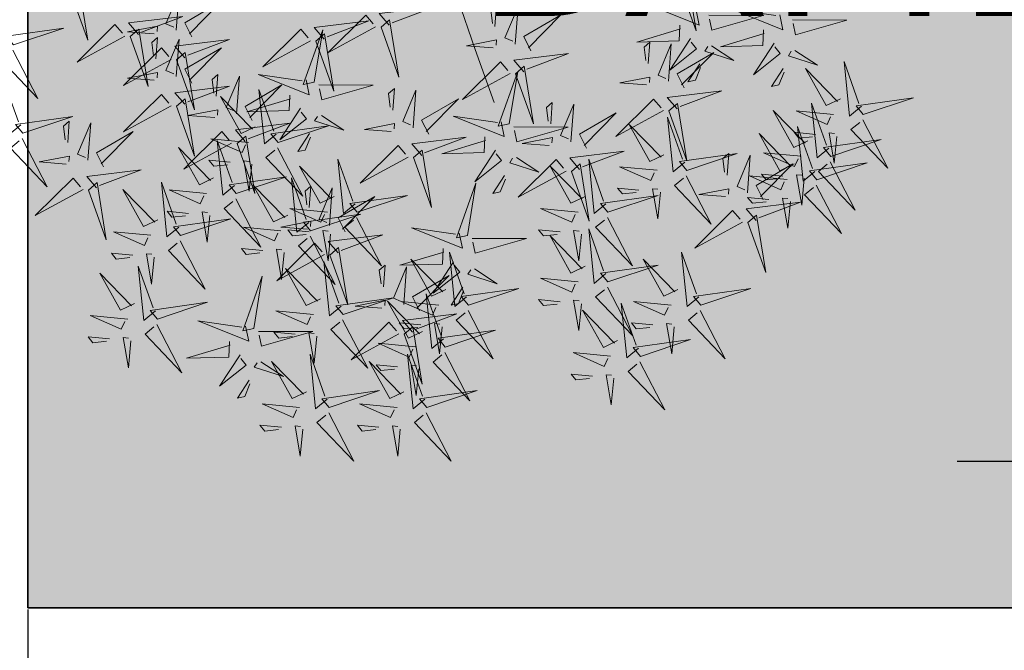
# Model space of a CAD drawing. Units: inches. Extents: x 1704 to 6393, y -157 to 1172.
# Tile 3 of 122: x 1898 to 1933, y -5 to 17. Entities that reach past the tile are written whole.
import ezdxf

# ---------------------------------------------------------------- set-up
doc = ezdxf.new("R2010")
doc.units = ezdxf.units.IN
doc.header["$MEASUREMENT"] = 0
for name, color, linetype, lineweight in [('A-ANNO-DIMS', 7, 'Continuous', 13), ('C-PROP', 7, 'Continuous', 35), ('L-shrub', 74, 'Continuous', 18), ('L-tree', 102, 'Continuous', 18)]:
    doc.layers.add(name, color=color, linetype=linetype, lineweight=lineweight)
doc.layers.add('L-PLNT-PATT', color=253, linetype='Continuous', lineweight=13, true_color=0x9abc8f)
doc.styles.get("Standard").update_dxf_attribs({"font": 'arial.ttf'})
doc.dimstyles.get("Standard").update_dxf_attribs({"dimtxt": 6, "dimasz": 2, "dimexe": 0.18, "dimexo": 0.0625, "dimgap": 0.09, "dimtad": 0, "dimtih": 1, "dimtoh": 1, "dimdec": 1, "dimzin": 0, "dimdsep": 46, "dimlunit": 3, "dimtxsty": 'Standard', "dimblk": 'ARCHTICK', "dimcen": 0.09, "dimadec": 0, "dimazin": 0, "dimtfac": 1, "dimtdec": 1, "dimtofl": 0, "dimtmove": 0, "dimatfit": 3, "dimfxl": 1, "dimtolj": 1, "dimtzin": 0, "dimarcsym": 0})

# ---------------------------------------------------------------- blocks, each defined once
blk = doc.blocks.new('bamboo')
blk.add_line((390, 162.3), (546.4, 218.1))
at = {"layer": 'L-shrub'}
blk.add_line((32.3, 39.5), (390, 162.3), dxfattribs=at)
for points in [[(581.6, 1302), (532.2, 1449.6), (555.7, 1280.7), (581.6, 1302)], [(597.3, 1300.4), (739.2, 1374), (625.7, 1265.9), (604.4, 1291.8)], [(704.4, 1206.5), (655.1, 1354.1), (678.6, 1185.2), (704.4, 1206.5)], [(772.7, 1165.6), (723.3, 1313.2), (746.9, 1144.3), (772.7, 1165.6)], [(557.2, 1296.4), (585.7, 1261.9), (425.4, 1245.7), (548.6, 1289.3)], [(720.2, 1205), (862.1, 1278.5), (748.6, 1170.5), (727.3, 1196.4)], [(303.5, 1094), (304.2, 1253.9), (347.3, 1103.2), (314.4, 1096.3)], [(535.5, 1235), (555.3, 1193.4), (446.4, 1132.5), (542.6, 1226.4)], [(581.2, 1214.7), (570.7, 1104.6), (611.1, 1195.9), (588.3, 1206.1)], [(645.6, 1224.3), (724.2, 1216.7), (635.4, 1201.5), (637, 1217.2)], [(788.4, 1164.1), (930.3, 1237.6), (816.9, 1129.6), (795.5, 1155.5)], [(680.1, 1200.9), (708.6, 1166.4), (548.3, 1150.2), (671.5, 1193.8)], [(393.3, 1101.5), (436.5, 1167.6), (408.8, 1082), (395.6, 1090.6)], [(748.4, 1160), (776.8, 1125.5), (616.6, 1109.3), (739.8, 1152.9)], [(639.6, 1161.5), (633.5, 1098.6), (650.8, 1112.8), (646.7, 1152.8)], [(658.4, 1139.6), (678.2, 1098), (569.2, 1037.1), (665.5, 1130.9)], [(768.4, 1128.9), (847.1, 1121.3), (758.3, 1106.1), (759.8, 1121.8)], [(726.6, 1098.6), (746.5, 1057), (637.5, 996.2), (733.8, 1090)], [(704, 1119.3), (693.5, 1009.2), (734, 1100.5), (711.2, 1110.6)], [(892.5, 987.3), (858.6, 958.2), (839.1, 1118), (885.2, 995.8)], [(830.7, 1007.8), (789.5, 987.1), (726.4, 1094.8), (822.2, 1000.5)], [(772.3, 1078.4), (761.8, 968.3), (802.3, 1059.6), (779.4, 1069.7)], [(836.7, 1088), (915.3, 1080.4), (826.6, 1065.2), (828.1, 1080.9)], [(288.5, 1056.7), (332.3, 1065.9), (272.3, 916.4), (290.8, 1045.7)], [(372, 1040), (464.6, 979.6), (402.5, 1057.8), (382.9, 1042.3)], [(446.2, 1067), (499.2, 1032.5), (494.6, 1054.4), (457.2, 1069.3)], [(762.4, 1066), (756.4, 1003.1), (773.6, 1017.3), (769.5, 1057.4)], [(830.7, 1025.1), (824.7, 962.2), (841.9, 976.4), (837.8, 1016.5)], [(898.5, 963.1), (1045.1, 1015.5), (876.7, 988.5), (898.5, 963.1)], [(289.9, 848.6), (290.5, 1008.4), (333.6, 857.8), (300.8, 850.9)], [(332.8, 1008.9), (378.9, 1007.2), (382.3, 882.5), (343.8, 1011.2)], [(811.3, 961.7), (701, 970), (793.1, 931.4), (802.8, 954.4)], [(1141.3, 824.7), (1092, 972.3), (1115.5, 803.4), (1141.3, 824.7)], [(745.4, 783.8), (696, 931.4), (719.6, 762.5), (745.4, 783.8)], [(897.3, 947.3), (973.8, 807), (863.4, 918.2), (888.9, 940.1)], [(379.6, 856.1), (422.9, 922.2), (395.2, 836.5), (381.9, 845.1)], [(759.2, 902.3), (696.2, 907), (710.8, 890.1), (750.8, 895)], [(822.2, 897.5), (816.2, 818.8), (799.2, 907.2), (815, 906)], [(1157.1, 823.2), (1299, 896.7), (1185.5, 788.7), (1164.2, 814.6)], [(564.8, 755.5), (530.9, 726.4), (511.4, 886.2), (557.5, 764)], [(503, 776), (461.8, 755.3), (398.7, 863), (494.5, 768.7)], [(761.1, 782.3), (903, 855.8), (789.6, 747.8), (768.2, 773.7)], [(188.6, 758.6), (335.2, 810.9), (166.8, 784), (188.6, 758.6)], [(274.9, 811.2), (318.6, 820.4), (258.7, 670.9), (277.2, 800.3)], [(358.3, 794.5), (451, 734.2), (388.8, 812.4), (369.3, 796.8)], [(432.6, 821.6), (485.5, 787.1), (480.9, 808.9), (443.5, 823.9)], [(1117, 819.1), (1145.4, 784.6), (985.2, 768.4), (1108.4, 812)], [(570.9, 731.3), (717.4, 783.7), (549, 756.7), (570.9, 731.3)], [(1291.5, 647.4), (1242.1, 795), (1265.7, 626.1), (1291.5, 647.4)], [(319.2, 763.5), (365.2, 761.8), (368.6, 637), (330.1, 765.8)], [(721.1, 778.2), (749.5, 743.7), (589.3, 727.5), (712.5, 771.1)], [(1095.3, 757.7), (1115.1, 716.2), (1006.1, 655.3), (1102.4, 749.1)], [(483.6, 729.9), (373.4, 738.2), (465.5, 699.6), (475.2, 722.6)], [(1140.9, 737.5), (1130.4, 627.4), (1170.9, 718.7), (1148, 728.8)], [(1205.3, 747.1), (1283.9, 739.5), (1195.2, 724.3), (1196.7, 740)], [(569.7, 715.5), (646.1, 575.2), (535.8, 686.4), (561.2, 708.3)], [(699.3, 716.8), (719.2, 675.2), (610.2, 614.4), (706.4, 708.2)], [(745, 696.6), (734.5, 586.5), (774.9, 677.8), (752.1, 687.9)], [(809.4, 706.2), (888, 698.6), (799.3, 683.4), (800.8, 699.1)], [(868.3, 552), (818.9, 699.6), (842.4, 530.7), (868.3, 552)], [(1073.1, 552), (1023.7, 699.6), (1047.2, 530.7), (1073.1, 552)], [(1307.2, 645.9), (1449.1, 719.5), (1335.7, 611.4), (1314.3, 637.3)], [(431.6, 670.5), (368.6, 675.2), (383.1, 658.2), (423.1, 663.2)], [(494.6, 665.7), (488.6, 587), (471.6, 675.4), (487.3, 674.2)], [(1199.3, 684.2), (1193.3, 621.3), (1210.5, 635.5), (1206.4, 675.6)], [(803.4, 643.3), (797.4, 580.4), (814.6, 594.6), (810.5, 634.7)], [(1267.2, 641.9), (1295.6, 607.4), (1135.4, 591.1), (1258.6, 634.8)], [(884, 550.5), (1025.9, 624), (912.4, 516), (891.1, 541.8)], [(1088.8, 550.5), (1230.7, 624), (1117.2, 516), (1095.9, 541.8)], [(742.3, 469.2), (708.4, 440), (688.9, 599.9), (735, 477.6)], [(1245.4, 580.5), (1265.3, 538.9), (1156.3, 478), (1252.6, 571.9)], [(680.5, 489.6), (639.3, 469), (576.2, 576.7), (672, 482.3)], [(1291.1, 560.2), (1280.6, 450.1), (1321.1, 541.4), (1298.2, 551.6)], [(1355.5, 569.8), (1434.1, 562.2), (1345.4, 547), (1346.9, 562.7)], [(843.9, 546.4), (872.4, 511.9), (712.1, 495.7), (835.3, 539.3)], [(1048.7, 546.4), (1077.2, 511.9), (916.9, 495.7), (1040.1, 539.3)], [(748.4, 444.9), (894.9, 497.3), (726.5, 470.3), (748.4, 444.9)], [(1349.5, 506.9), (1343.5, 444), (1360.7, 458.2), (1356.6, 498.3)], [(822.2, 485), (842, 443.4), (733.1, 382.6), (829.3, 476.4)], [(867.9, 464.7), (857.4, 354.7), (897.8, 446), (875, 456.1)], [(932.3, 474.4), (1010.9, 466.8), (922.2, 451.6), (923.7, 467.3)], [(1027, 485), (1046.8, 443.4), (937.9, 382.6), (1034.1, 476.4)], [(1072.7, 464.7), (1062.1, 354.7), (1102.6, 446), (1079.8, 456.1)], [(1137.1, 474.4), (1215.7, 466.8), (1126.9, 451.6), (1128.4, 467.3)], [(455.6, 305.5), (421.7, 276.4), (402.2, 436.3), (448.3, 314)], [(661.1, 443.6), (550.9, 451.8), (643, 413.2), (652.6, 436.3)], [(617.5, 275.9), (618.2, 435.7), (661.3, 285.1), (628.5, 278.2)], [(393.8, 326), (352.6, 305.3), (289.5, 413), (385.3, 318.7)], [(747.2, 429.2), (823.6, 288.8), (713.3, 400), (738.7, 421.9)], [(926.3, 411.5), (920.3, 348.6), (937.5, 362.8), (933.4, 402.9)], [(1131.1, 411.5), (1125, 348.6), (1142.3, 362.8), (1138.2, 402.9)], [(609.1, 384.1), (546.1, 388.8), (560.6, 371.9), (600.6, 376.8)], [(672.1, 379.4), (666.1, 300.6), (649, 389), (664.8, 387.8)], [(707.3, 283.4), (750.5, 349.5), (722.8, 263.8), (709.6, 272.4)], [(461.7, 281.3), (608.2, 333.7), (439.8, 306.7), (461.7, 281.3)], [(945.2, 153.2), (945.8, 313), (988.9, 162.4), (956.1, 155.5)], [(1141.3, 142.9), (1092, 290.5), (1115.5, 121.6), (1141.3, 142.9)], [(374.4, 279.9), (264.1, 288.2), (356.3, 249.6), (365.9, 272.6)], [(460.4, 265.6), (536.9, 125.2), (426.5, 236.4), (452, 258.3)], [(608.9, 262.7), (455.2, 287.4), (615.8, 229.9), (608.9, 262.7)], [(602.5, 238.5), (646.3, 247.7), (586.3, 98.2), (604.8, 227.6)], [(686, 221.8), (778.6, 161.5), (716.5, 239.7), (696.9, 224.1)], [(760.2, 248.9), (813.2, 214.4), (808.6, 236.2), (771.2, 251.2)], [(322.4, 220.5), (259.3, 225.2), (273.9, 208.3), (313.9, 213.2)], [(385.4, 215.7), (379.4, 137), (362.3, 225.4), (378.1, 224.2)], [(1035, 160.6), (1078.2, 226.8), (1050.5, 141.1), (1037.3, 149.7)], [(1157.1, 141.4), (1299, 214.9), (1185.5, 106.9), (1164.2, 132.8)], [(1264.2, 74.7), (1214.8, 222.3), (1238.4, 53.4), (1264.2, 74.7)], [(646.8, 190.8), (692.9, 189.1), (696.3, 64.3), (657.8, 193.1)], [(936.5, 139.9), (782.9, 164.7), (943.4, 107.2), (936.5, 139.9)], [(1279.9, 73.2), (1421.8, 146.8), (1308.4, 38.7), (1287, 64.6)], [(1441.7, 20.2), (1392.3, 167.8), (1415.9, -1.1), (1441.7, 20.2)], [(701.3, 5.5), (667.4, -23.6), (647.9, 136.3), (694, 14)], [(930.2, 115.8), (973.9, 125), (914, -24.5), (932.5, 104.9)], [(1117, 137.3), (1145.4, 102.8), (985.2, 86.6), (1108.4, 130.2)], [(1013.6, 99.1), (1106.3, 38.8), (1044.2, 116.9), (1024.6, 101.4)], [(1087.9, 126.1), (1140.9, 91.6), (1136.3, 113.5), (1098.9, 128.4)], [(639.5, 26), (598.3, 5.3), (535.3, 113), (631, 18.7)], [(1220.1, -21.7), (1186.2, -50.9), (1166.7, 109), (1212.8, -13.3)], [(1457.4, 18.7), (1599.3, 92.2), (1485.9, -15.8), (1464.5, 10)], [(974.5, 68.1), (1020.5, 66.3), (1023.9, -58.4), (985.4, 70.4)], [(1095.3, 76), (1115.1, 34.4), (1006.1, -26.5), (1102.4, 67.3)], [(1158.3, -1.3), (1117.1, -21.9), (1054.1, 85.8), (1149.8, -8.5)], [(1239.9, 69.2), (1268.3, 34.7), (1108.1, 18.4), (1231.3, 62.1)], [(1205.3, 65.3), (1283.9, 57.7), (1195.2, 42.5), (1196.7, 58.2)], [(319, -89.9), (285.1, -119.1), (265.6, 40.8), (311.8, -81.4)], [(707.4, -18.7), (854, 33.7), (685.6, 6.7), (707.4, -18.7)], [(1140.9, 55.7), (1130.4, -54.4), (1170.9, 36.9), (1148, 47)], [(1218.1, 7.8), (1238, -33.8), (1129, -94.7), (1225.2, -0.8)], [(1199.3, 2.4), (1193.3, -60.5), (1210.5, -46.3), (1206.4, -6.2)], [(1226.2, -46), (1372.8, 6.4), (1204.4, -20.6), (1226.2, -46)], [(1417.4, 14.6), (1445.8, -19.9), (1285.6, -36.1), (1408.7, 7.5)], [(620.2, -20.1), (509.9, -11.8), (602, -50.4), (611.7, -27.3)], [(1263.8, -12.5), (1253.3, -122.6), (1293.7, -31.3), (1270.9, -21.1)], [(1328.2, -2.9), (1406.8, -10.5), (1318.1, -25.7), (1319.6, -10)], [(706.2, -34.4), (782.6, -174.8), (672.3, -63.6), (697.7, -41.7)], [(868.3, -184.3), (818.9, -36.7), (842.4, -205.6), (868.3, -184.3)], [(1139, -47.3), (1028.7, -39.1), (1120.8, -77.6), (1130.5, -54.6)], [(1395.6, -46.8), (1415.5, -88.4), (1306.5, -149.2), (1402.7, -55.4)], [(1505.7, -57.4), (1584.3, -65), (1495.6, -80.2), (1497.1, -64.5)], [(325.1, -114.1), (471.7, -61.8), (303.3, -88.7), (325.1, -114.1)], [(568.1, -79.5), (505.1, -74.8), (519.6, -91.7), (559.6, -86.8)], [(631.1, -84.2), (625.1, -163), (608.1, -74.6), (623.8, -75.8)], [(1168.6, -225.3), (1119.3, -77.6), (1142.8, -246.6), (1168.6, -225.3)], [(1225, -61.7), (1301.4, -202.1), (1191.1, -90.8), (1216.5, -69)], [(1322.2, -65.8), (1316.2, -128.7), (1333.4, -114.5), (1329.3, -74.4)], [(1441.3, -67.1), (1430.8, -177.1), (1471.2, -85.8), (1448.4, -75.7)], [(884, -185.9), (1025.9, -112.3), (912.4, -220.4), (891.1, -194.5)], [(988, -239.9), (954.1, -269), (934.6, -109.2), (980.8, -231.4)], [(1086.9, -106.8), (1023.9, -102.1), (1038.4, -119), (1078.4, -114.1)], [(1149.9, -111.5), (1143.9, -190.3), (1126.9, -101.9), (1142.6, -103)], [(323.9, -129.9), (400.4, -270.3), (290, -159), (315.4, -137.2)], [(494.6, -296.8), (495.3, -137), (538.4, -287.6), (505.6, -294.5)], [(926.2, -219.4), (885, -240.1), (822, -132.4), (917.7, -226.7)], [(1441.7, -266.2), (1392.3, -118.6), (1415.9, -287.5), (1441.7, -266.2)], [(1499.7, -120.3), (1493.7, -183.2), (1510.9, -169), (1506.8, -128.9)], [(360, -280.8), (326.1, -310), (306.6, -150.1), (352.7, -272.3)], [(922.9, -320.7), (873.5, -173.1), (897.1, -342), (922.9, -320.7)], [(1184.4, -226.8), (1326.3, -153.2), (1212.8, -261.3), (1191.5, -235.4)], [(843.9, -189.9), (872.4, -224.4), (712.1, -240.6), (835.3, -197)], [(1457.4, -267.7), (1599.3, -194.1), (1485.9, -302.2), (1464.5, -276.3)], [(584.4, -289.3), (627.6, -223.2), (600, -308.9), (586.7, -300.3)], [(994.1, -264.1), (1140.7, -211.8), (972.3, -238.7), (994.1, -264.1)], [(1144.3, -230.8), (1172.7, -265.3), (1012.5, -281.6), (1135.7, -237.9)], [(366.1, -305), (512.7, -252.7), (344.3, -279.6), (366.1, -305)], [(822.2, -251.3), (842, -292.9), (733.1, -353.8), (829.3, -259.9)], [(906.9, -265.5), (796.6, -257.2), (888.7, -295.8), (898.4, -272.8)], [(938.6, -322.2), (1080.5, -248.7), (967.1, -356.7), (945.7, -330.8)], [(486, -310), (332.3, -285.3), (492.9, -342.8), (486, -310)], [(663.5, -416.2), (614.1, -268.5), (637.6, -437.5), (663.5, -416.2)], [(867.9, -271.6), (857.4, -381.7), (897.8, -290.4), (875, -280.2)], [(932.3, -262), (1010.9, -269.6), (922.2, -284.8), (923.7, -269.1)], [(992.9, -279.9), (1069.3, -420.3), (959, -309), (984.4, -287.2)], [(1417.4, -271.7), (1445.8, -306.2), (1285.6, -322.5), (1408.7, -278.8)], [(1122.6, -292.2), (1142.4, -333.8), (1033.4, -394.7), (1129.7, -300.8)], [(1168.2, -312.5), (1157.7, -422.6), (1198.2, -331.3), (1175.3, -321.1)], [(1218.2, -474.1), (1218.9, -314.2), (1262, -464.9), (1229.2, -471.8)], [(1232.6, -302.9), (1311.2, -310.5), (1222.5, -325.7), (1224, -310)], [(364.9, -320.8), (441.3, -461.2), (331, -349.9), (356.4, -328.1)], [(479.7, -334.2), (523.4, -325), (463.5, -474.5), (482, -345.1)], [(563.1, -350.9), (655.8, -411.2), (593.6, -333), (574, -348.6)], [(637.4, -323.8), (690.3, -358.3), (685.7, -336.5), (648.3, -321.5)], [(679.2, -417.7), (821.1, -344.1), (707.7, -452.2), (686.3, -426.3)], [(898.6, -326.3), (927, -360.8), (766.8, -377), (889.9, -333.4)], [(854.8, -325), (791.8, -320.2), (806.4, -337.2), (846.3, -332.2)], [(917.8, -329.7), (911.8, -408.4), (894.8, -320), (910.5, -321.2)], [(926.3, -324.9), (920.3, -387.8), (937.5, -373.5), (933.4, -333.5)], [(1395.6, -333.1), (1415.5, -374.7), (1306.5, -435.6), (1402.7, -341.7)], [(1505.7, -343.8), (1584.3, -351.4), (1495.6, -366.6), (1497.1, -350.9)], [(1226.6, -365.8), (1220.6, -428.7), (1237.8, -414.5), (1233.7, -374.4)], [(1441.3, -353.4), (1430.8, -463.5), (1471.2, -372.2), (1448.4, -362)], [(524, -381.9), (570, -383.6), (573.4, -508.4), (534.9, -379.6)], [(660.4, -512.6), (626.5, -541.8), (607, -381.9), (653.1, -504.2)], [(813.7, -538.9), (764.3, -391.3), (787.8, -560.2), (813.7, -538.9)], [(876.8, -387.7), (896.6, -429.3), (787.7, -490.1), (883.9, -396.3)], [(986.9, -398.3), (1065.5, -405.9), (976.8, -421.1), (978.3, -405.4)], [(1308, -466.6), (1351.2, -400.5), (1323.6, -486.2), (1310.3, -477.5)], [(598.6, -492.1), (557.4, -512.8), (494.3, -405.1), (590.1, -499.4)], [(639.2, -421.7), (667.6, -456.2), (507.4, -472.5), (630.5, -428.8)], [(922.5, -407.9), (912, -518), (952.4, -426.7), (929.6, -416.6)], [(1499.7, -406.7), (1493.7, -469.6), (1510.9, -455.4), (1506.8, -415.3)], [(980.9, -461.2), (974.9, -524.1), (992.1, -509.9), (988, -469.8)], [(617.4, -483.1), (637.2, -524.7), (528.3, -585.6), (624.5, -491.7)], [(666.4, -536.8), (813, -484.5), (644.6, -511.4), (666.4, -536.8)], [(829.4, -540.4), (971.3, -466.8), (857.8, -574.9), (836.5, -549)], [(1209.6, -487.3), (1055.9, -462.6), (1216.5, -520.1), (1209.6, -487.3)], [(663.1, -503.4), (652.6, -613.5), (693, -522.2), (670.2, -512)], [(727.5, -493.8), (806.1, -501.4), (717.4, -516.6), (718.9, -500.9)], [(1203.3, -511.5), (1247, -502.3), (1187.1, -651.7), (1205.5, -522.4)], [(1286.7, -528.1), (1379.3, -588.5), (1317.2, -510.3), (1297.6, -525.8)], [(1361, -501.1), (1413.9, -535.6), (1409.3, -513.8), (1371.9, -498.8)], [(579.2, -538.2), (468.9, -529.9), (561.1, -568.5), (570.7, -545.5)], [(789.3, -544.5), (817.8, -578.9), (657.5, -595.2), (780.7, -551.6)], [(414.6, -689.9), (380.7, -719), (361.2, -559.2), (407.3, -681.4)], [(551.1, -689.9), (517.2, -719), (497.7, -559.2), (543.9, -681.4)], [(665.2, -552.6), (741.7, -693), (631.3, -581.7), (656.8, -559.9)], [(721.5, -556.7), (715.5, -619.6), (732.7, -605.4), (728.6, -565.3)], [(936.5, -702.5), (887.2, -554.9), (910.7, -723.8), (936.5, -702.5)], [(1247.5, -559.2), (1293.6, -560.9), (1297, -685.7), (1258.5, -556.9)], [(352.8, -669.4), (311.6, -690.1), (248.5, -582.4), (344.3, -676.7)], [(489.3, -669.4), (448.2, -690.1), (385.1, -582.4), (480.9, -676.7)], [(527.1, -597.7), (464.1, -593), (478.7, -609.9), (518.7, -605)], [(590.2, -602.4), (584.1, -681.2), (567.1, -592.8), (582.9, -593.9)], [(767.6, -605.8), (787.4, -647.4), (678.5, -708.3), (774.7, -614.5)], [(813.3, -626.1), (802.7, -736.2), (843.2, -644.9), (820.4, -634.7)], [(877.7, -616.5), (956.3, -624.1), (867.5, -639.3), (869, -623.6)], [(952.3, -704), (1094.2, -630.5), (980.7, -738.5), (959.4, -712.7)], [(1182.3, -770.7), (1132.9, -623.1), (1156.5, -792), (1182.3, -770.7)], [(420.7, -714.1), (567.3, -661.7), (398.9, -688.7), (420.7, -714.1)], [(557.2, -714.1), (703.8, -661.7), (535.4, -688.7), (557.2, -714.1)], [(871.6, -679.4), (865.6, -742.3), (882.9, -728.1), (878.8, -688)], [(333.5, -715.5), (223.2, -707.2), (315.3, -745.8), (325, -722.8)], [(346.4, -826.2), (312.4, -855.4), (293, -695.5), (339.1, -817.8)], [(470, -715.5), (359.7, -707.2), (451.8, -745.8), (461.5, -722.8)], [(912.2, -708.1), (940.6, -742.6), (780.4, -758.8), (903.6, -715.2)], [(1198, -772.2), (1339.9, -698.7), (1226.5, -806.7), (1205.1, -780.8)], [(419.5, -729.9), (495.9, -870.2), (385.6, -759), (411, -737.1)], [(556, -729.9), (632.4, -870.2), (522.1, -759), (547.5, -737.1)], [(344.4, -779.7), (338.4, -858.4), (321.4, -770), (337.1, -771.2)], [(417.9, -774.9), (354.9, -770.2), (369.5, -787.1), (409.4, -782.2)], [(480.9, -779.7), (474.9, -858.4), (457.9, -770), (473.7, -771.2)], [(890.5, -769.5), (910.3, -811.1), (801.3, -871.9), (897.6, -778.1)], [(1000.5, -780.1), (1079.1, -787.7), (990.4, -802.9), (991.9, -787.2)], [(1158, -776.3), (1186.4, -810.8), (1026.2, -827), (1149.3, -783.4)], [(352.4, -850.5), (499, -798.1), (330.6, -825.1), (352.4, -850.5)], [(936.1, -789.8), (925.6, -899.8), (966.1, -808.5), (943.2, -798.4)], [(796.9, -949), (763, -978.1), (743.5, -818.2), (789.6, -940.5)], [(1136.2, -837.6), (1156, -879.2), (1047.1, -940.1), (1143.3, -846.3)], [(351.2, -866.2), (427.7, -1006.6), (317.3, -895.4), (342.8, -873.5)], [(735.1, -928.5), (693.9, -949.2), (630.8, -841.5), (726.6, -935.8)], [(994.5, -843), (988.5, -905.9), (1005.7, -891.7), (1001.6, -851.6)], [(1181.9, -857.9), (1171.4, -968), (1211.8, -876.7), (1189, -866.6)], [(1246.3, -848.3), (1324.9, -855.9), (1236.2, -871.1), (1237.7, -855.4)], [(803, -973.2), (949.5, -920.8), (781.1, -947.8), (803, -973.2)], [(1240.3, -911.2), (1234.3, -974.1), (1251.5, -959.9), (1247.4, -919.8)], [(215.9, -1027.7), (362.5, -975.4), (194.1, -1002.3), (215.9, -1027.7)], [(715.7, -974.6), (605.5, -966.3), (697.6, -1004.9), (707.3, -981.8)], [(801.8, -988.9), (878.2, -1129.3), (767.9, -1018.1), (793.3, -996.2)], [(636.2, -1166.1), (586.8, -1018.5), (610.3, -1187.4), (636.2, -1166.1)], [(663.7, -1034), (600.7, -1029.3), (615.2, -1046.2), (655.2, -1041.3)], [(726.7, -1038.7), (720.7, -1117.5), (703.7, -1029.1), (719.4, -1030.3)], [(376.8, -1193.4), (327.4, -1045.8), (350.9, -1214.7), (376.8, -1193.4)], [(651.9, -1167.6), (793.8, -1094.1), (680.3, -1202.1), (659, -1176.3)], [(392.5, -1194.9), (534.4, -1121.4), (420.9, -1229.4), (399.6, -1203.5)], [(611.8, -1171.7), (640.3, -1206.2), (480.1, -1222.4), (603.2, -1178.8)]]:
    blk.add_lwpolyline(points, dxfattribs=at)
blk = doc.blocks.new('_ArchTick')
at = {"color": 0, "linetype": 'ByBlock', "const_width": 0.15}
blk.add_lwpolyline([(-0.5, -0.5), (0.5, 0.5)], dxfattribs=at)
blk = doc.blocks.new('*D70')
at = {"layer": 'A-ANNO-DIMS', "color": 0, "lineweight": -2, "transparency": 16777216}
for p, q in [((1931.245, 38.926), (1936.991, 38.926)), ((1936.811, 38.926), (1936.811, 23.36)), ((1936.811, 1.402), (1936.811, 16.968)), ((1931.245, 1.402), (1936.991, 1.402))]:
    blk.add_line(p, q, dxfattribs=at)
at = {"layer": 'Defpoints', "color": 0, "lineweight": -3, "transparency": 16777216}
for p in [(1931.183, 38.926), (1931.183, 1.402), (1936.811, 1.402)]:
    blk.add_point(p, dxfattribs=at)
at = {"layer": 'A-ANNO-DIMS', "color": 0, "lineweight": -2, "transparency": 16777216, "xscale": 2, "yscale": 2, "zscale": 2}
for p, rotation in [((1936.811, 38.926), 90), ((1936.811, 1.402), 270)]:
    blk.add_blockref('_ArchTick', p, dxfattribs=dict(at, rotation=rotation))
at = {"layer": 'A-ANNO-DIMS', "color": 0, "transparency": 16777216, "insert": (1936.811, 20.164), "char_height": 6, "attachment_point": 5}
blk.add_mtext('\\A1;BAMBOO 38', dxfattribs=at)
blk = doc.blocks.new('*D90')
at = {"layer": 'A-ANNO-DIMS', "color": 0, "lineweight": -2, "transparency": 16777216}
for p, q in [((1898.349, -3.85), (1898.349, -64.967)), ((2723.349, -3.85), (2723.349, -64.967)), ((1898.349, -64.787), (2304.104, -64.787)), ((2723.349, -64.787), (2317.593, -64.787))]:
    blk.add_line(p, q, dxfattribs=at)
at = {"layer": 'Defpoints', "color": 0, "lineweight": -3, "transparency": 16777216}
for p in [(1898.349, -3.787), (2723.349, -3.787), (2723.349, -64.787)]:
    blk.add_point(p, dxfattribs=at)
at = {"layer": 'A-ANNO-DIMS', "color": 0, "lineweight": -2, "transparency": 16777216, "xscale": 2, "yscale": 2, "zscale": 2, "rotation": 180}
blk.add_blockref('_ArchTick', (1898.349, -64.787), dxfattribs=at)
at = {"layer": 'A-ANNO-DIMS', "color": 0, "lineweight": -2, "transparency": 16777216, "xscale": 2, "yscale": 2, "zscale": 2}
blk.add_blockref('_ArchTick', (2723.349, -64.787), dxfattribs=at)
at = {"layer": 'A-ANNO-DIMS', "color": 0, "transparency": 16777216, "insert": (2310.849, -64.787), "char_height": 6, "attachment_point": 5}
blk.add_mtext('\\A1;825', dxfattribs=at)

msp = doc.modelspace()

# ---------------------------------------------------------------- hatches: boundary and pattern name
at = {"layer": 'L-PLNT-PATT', "transparency": 33554643}
h = msp.add_hatch(color=256, dxfattribs=at)
h.dxf.hatch_style = 1
h.paths.add_polyline_path([(1975.349, 202.213), (1898.349, 202.213), (1898.349, -3.787), (1975.349, -3.787)])

# ---------------------------------------------------------------- linework, layer by layer
at = {"layer": 'C-PROP'}
for p, q in [((1898.349, -3.787), (1898.349, 1033.213)), ((2723.349, -3.787), (1898.349, -3.787))]:
    msp.add_line(p, q, dxfattribs=at)

# ---------------------------------------------------------------- block references
at = {"layer": 'L-tree', "xscale": 0.0120554306156665, "yscale": 0.0120554306156665, "zscale": 0.0120554306156665, "rotation": 270}
msp.add_blockref('bamboo', (1912.228, 20.683), dxfattribs=at)

# ---------------------------------------------------------------- dimensions: what is measured, and where the dimension line sits
at = {"layer": 'A-ANNO-DIMS'}
dim = msp.add_linear_dim(base=(1936.811, 1.402), p1=(1931.183, 38.926), p2=(1931.183, 1.402), angle=270, text='BAMBOO <>', dimstyle='Standard', override={"dimdec": 0, "dimlfac": 1, "dimrnd": 0, "dimzin": 0, "dimdsep": 46, "dimlunit": 2}, dxfattribs=at)
dim.commit()
dim.dimension.update_dxf_attribs({"geometry": '*D70', "text_midpoint": (1936.811, 20.164)})
dim = msp.add_linear_dim(base=(2723.349, -64.787), p1=(1898.349, -3.787), p2=(2723.349, -3.787), dimstyle='Standard', override={"dimdec": 0, "dimlfac": 1, "dimrnd": 0, "dimzin": 0, "dimdsep": 46, "dimlunit": 2}, dxfattribs=at)
dim.commit()
dim.dimension.update_dxf_attribs({"geometry": '*D90', "text_midpoint": (2310.849, -64.787)})

doc.saveas('drawing.dxf')
